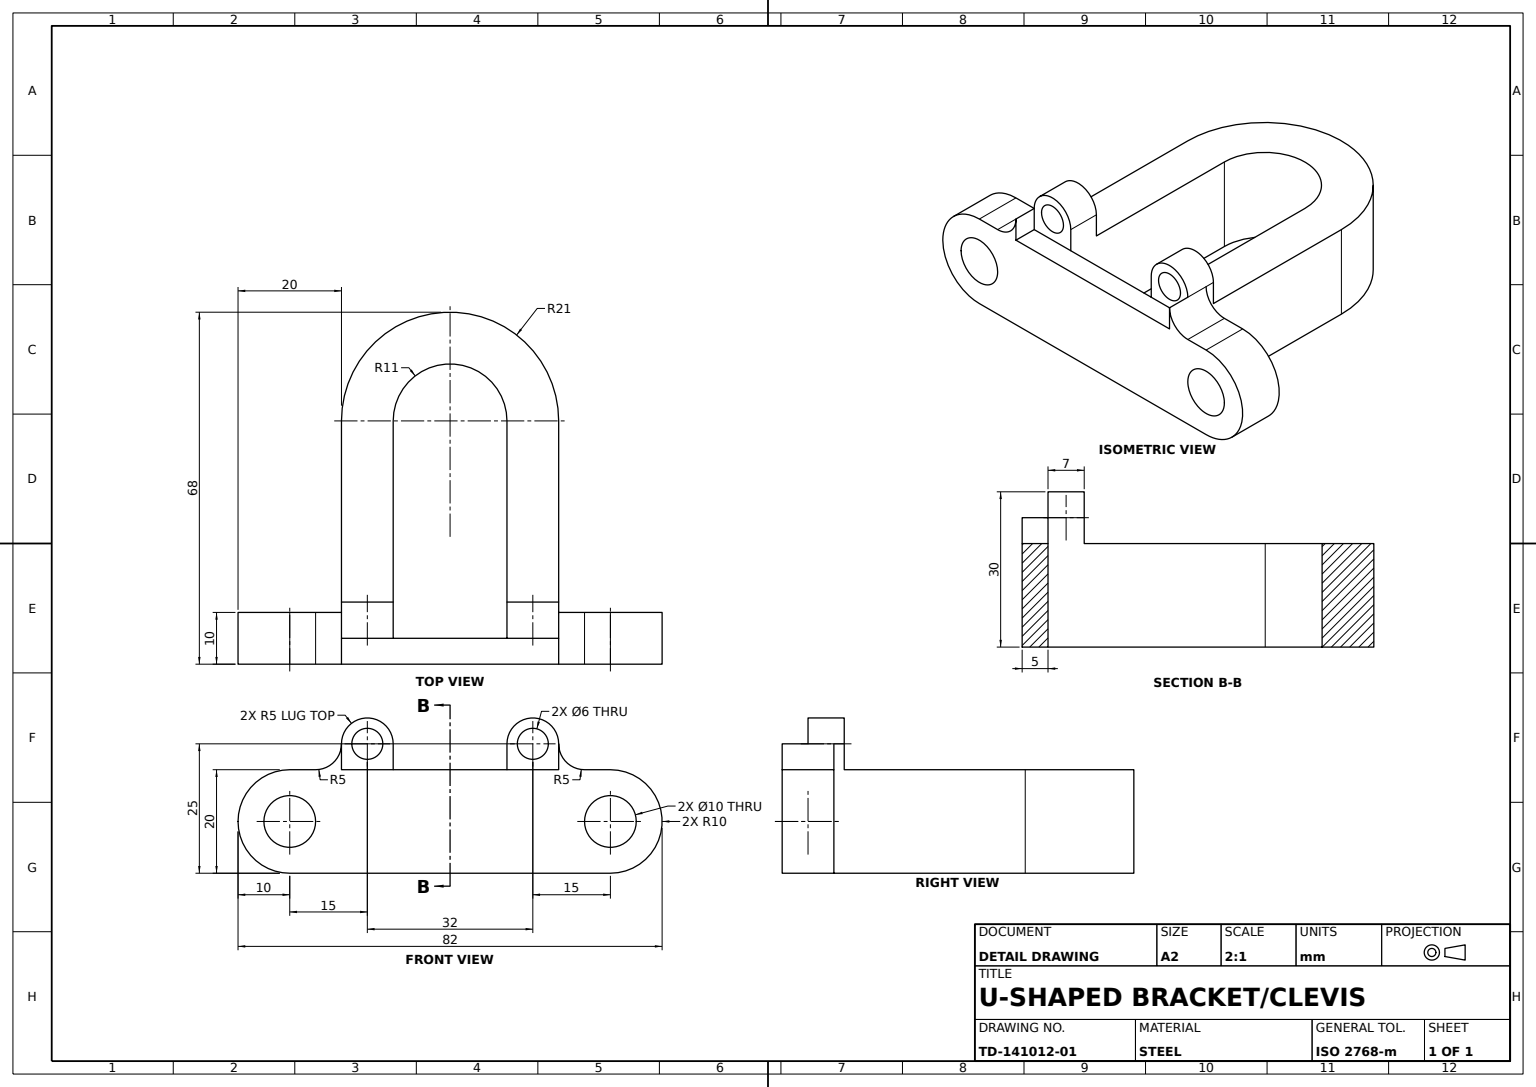
SolidWorks part; units mm, degrees
material "Plain Carbon Steel"
ref_plane "Front Plane" through (0, 0, 0) normal (0, 0, 1) x (1, 0, 0)
ref_plane "Top Plane" through (0, 0, 0) normal (0, 1, 0) x (1, 0, 0)
ref_plane "Right Plane" through (0, 0, 0) normal (1, 0, 0) x (0, 0, -1)
sketch "Base Plate Sketch" plane through (0, 0, 0) normal (0, 0, 1) x (1, 0, 0)
  line L0 (0, 0) -> (42, 0)
  line L1 (42, 0) -> (42, 20)
  line L2 (42, 20) -> (0, 20)
  line L3 (0, 20) -> (0, 0)
  dimension "D1" = 42
  dimension "D2" = 20
extrude "Base Plate" add sketch "Base Plate Sketch" along normal blind 5
ref_plane "Plane6" through (0, 20, 0) normal (0, 1, 0) x (1, 0, 0)
sketch "Curved Loop Sketch" plane through (0, 20, 0) normal (0, 1, 0) x (1, 0, 0)
  line L0 (21, 0) -> (21, 42) construction
  line L1 (42, 0) -> (0, 0) construction
  line L2 (0, 42) -> (0, 0)
  line L3 (0, 0) -> (42, 0)
  line L4 (42, 0) -> (42, 42)
  arc A0 (42, 42) -> (0, 42) centre (21, 42) ccw
  dimension "D1" = 42
extrude "Curved Loop Boss" add sketch "Curved Loop Sketch" against normal through all
sketch "Loop Slot Sketch" plane through (0, 20, 0) normal (0, 1, 0) x (1, 0, 0)
  line L0 (10, 42) -> (10, 0)
  line L1 (10, 0) -> (32, 0)
  line L2 (32, 0) -> (32, 42)
  arc A0 (32, 42) -> (10, 42) centre (21, 42) ccw
  dimension "D1" = 22
extrude "Loop Slot Cut" cut sketch "Loop Slot Sketch" against normal through all
ref_plane "Plane12" through (0, 0, 0) normal (0, 0, 1) x (1, 0, 0)
sketch "Lug Sketch" plane through (0, 0, 0) normal (0, 0, 1) x (1, 0, 0)
  line L0 (0, 20) -> (5, 20) construction
  line L1 (42, 20) -> (0, 20) construction
  line L2 (5, 20) -> (5, 25) construction
  line L3 (0, 25) -> (0, 20)
  line L4 (0, 20) -> (10, 20)
  line L5 (10, 20) -> (10, 25)
  arc A0 (10, 25) -> (0, 25) centre (5, 25) ccw
  circle A1 centre (5, 25) radius 3
  dimension "D1" = 6
  dimension "D2" = 5
extrude "Lug Boss" add sketch "Lug Sketch" against normal blind 7
ref_plane "Plane13" through (21, 0, 0) normal (1, 0, 0) x (0, 0, -1)
mirror "Lug Mirror" about plane through (21, 0, 0) normal (1, 0, 0) of "Lug Boss"
ref_plane "Plane14" through (0, 0, 0) normal (0, 0, 1) x (1, 0, 0)
sketch "Pin Eye Sketch" plane through (0, 0, 0) normal (0, 0, 1) x (1, 0, 0)
  line L0 (0, 10) -> (-10, 10) construction
  line L1 (0, 20) -> (0, 0) construction
  line L2 (-10, 20) -> (-5, 20)
  line L3 (0, 20) -> (0, 0)
  line L4 (0, 0) -> (-10, 0)
  line L5 (0, 25) -> (0, 20)
  arc A0 (-10, 20) -> (-10, 0) centre (-10, 10) ccw
  circle A1 centre (-10, 10) radius 5
  arc A2 (-5, 20) -> (0, 25) centre (-5, 25) ccw
  dimension "D1" = 10
  dimension "D2" = 10
extrude "Pin Eye Boss" add sketch "Pin Eye Sketch" along normal mid plane 10
ref_plane "Plane16" through (21, 0, 0) normal (1, 0, 0) x (0, 0, -1)
mirror "Pin Eye Mirror" about plane through (21, 0, 0) normal (1, 0, 0) of "Pin Eye Boss"
